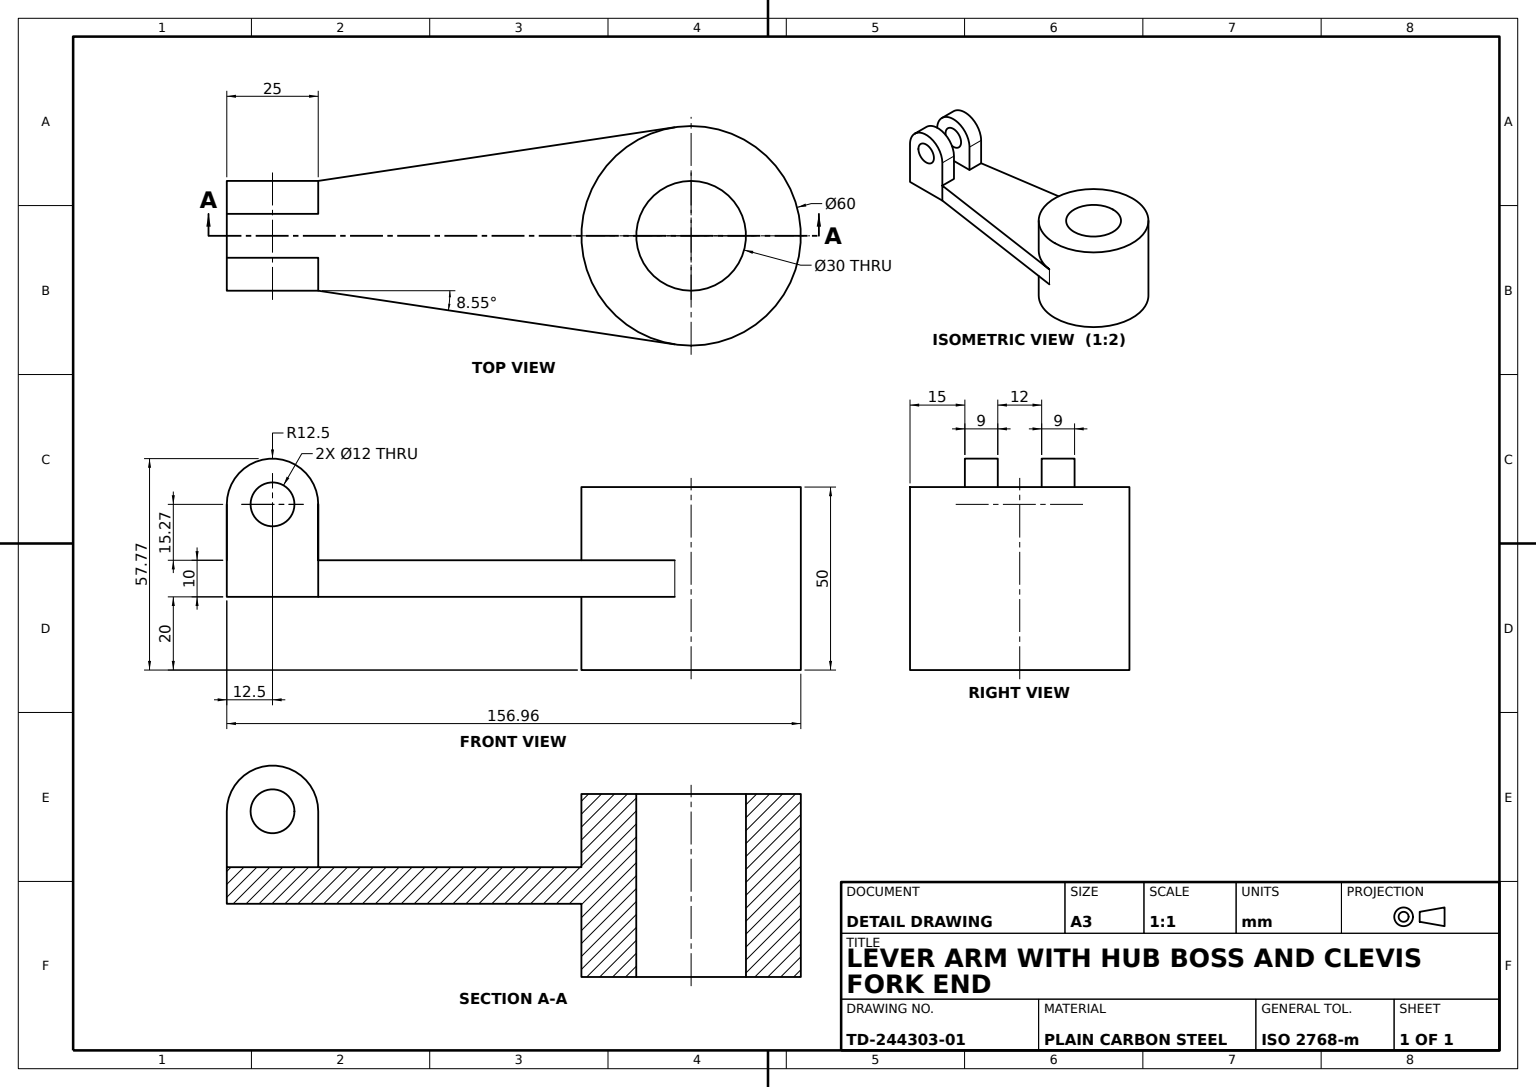
SolidWorks part; units mm, degrees
material "Plain Carbon Steel"
ref_plane "Front Plane" through (0, 0, 0) normal (0, 0, 1) x (1, 0, 0)
ref_plane "Top Plane" through (0, 0, 0) normal (0, 1, 0) x (1, 0, 0)
ref_plane "Right Plane" through (0, 0, 0) normal (1, 0, 0) x (0, 0, -1)
sketch "Hub Sketch Ø60" plane through (0, 0, 0) normal (0, 1, 0) x (1, 0, 0)
  circle A0 centre (0, 0) radius 30
  dimension "D1" = 60
extrude "Hub Ø60x50" add sketch "Hub Sketch Ø60" along normal mid plane 50
sketch "Bore Sketch Ø30" plane through (0, 25, 0) normal (0, 1, 0) x (1, 0, 0)
  circle A0 centre (0, 0) radius 15
  dimension "D1" = 30
extrude "Hub Bore Ø30" cut sketch "Bore Sketch Ø30" against normal through all contours A0
sketch "Arm Plate Sketch" plane through (0, 0, 0) normal (0, 1, 0) x (1, 0, 0)
  line L0 (-101.9625, 15) -> (-4.4625, 29.6662)
  line L1 (-101.9625, -15) -> (-4.4625, -29.6662)
  line L2 (-101.9625, -15) -> (-101.9625, 15)
  arc A0 (-4.4625, 29.6662) -> (-4.4625, -29.6662) centre (0, 0) ccw
  dimension "D1" = 60
  dimension "D2" = 97.5
  dimension "D3" = 30
  dimension "D4" = 97.5
extrude "Arm Plate 10mm" add sketch "Arm Plate Sketch" along normal mid plane 10 contours L2 L0 A0 L1
sketch "Clevis Base Sketch" plane through (0, 5, 0) normal (0, 1, 0) x (1, 0, 0)
  line L0 (-101.9625, -15) -> (-126.9625, -15)
  line L1 (-126.9625, -15) -> (-126.9625, 15)
  line L2 (-101.9625, 15) -> (-126.9625, 15)
  line L6 (-101.9625, -15) -> (-4.4625, -29.6662)
  line L7 (-4.4625, 29.6662) -> (-101.9625, 15)
  line L8 (-101.9625, 15) -> (-101.9625, -15)
  line L9 (-101.9625, -15) -> (-4.4625, -29.6662)
  line L10 (-4.4625, 29.6662) -> (-101.9625, 15)
  arc A1 (-4.4625, 29.6662) -> (-4.4625, -29.6662) centre (0, 0) ccw
  arc A2 (-4.4625, 29.6662) -> (-4.4625, -29.6662) centre (0, 0) ccw
  dimension "D1" = 25
  dimension "D2" = 0
extrude "Clevis Base" add sketch "Clevis Base Sketch" against normal blind 10 contours L0 L1 L2 L10 A2 L9
sketch "Clevis Lug 1 Sketch" plane through (0, 0, 15) normal (0, 0, 1) x (1, 0, 0)
  line L0 (-101.9625, 5) -> (-101.9625, 20.2721)
  line L1 (-126.9625, -5) -> (-126.9625, 5) construction
  line L2 (-126.9625, 20.2721) -> (-126.9625, 5)
  line L4 (-101.9625, 5) -> (-126.9625, 5) construction
  arc A0 (-101.9625, 20.2721) -> (-126.9625, 20.2721) centre (-114.4625, 20.2721) ccw
  circle A1 centre (-114.4625, 20.2721) radius 6
  line M1 (-101.9625, 5) -> (-126.9625, 5)
  dimension "D1" = 12
  dimension "D2" = 15.2721
extrude "Clevis Lug 1" add sketch "Clevis Lug 1 Sketch" against normal blind 9 contours L0 A0 L2 A1 M1
sketch "Clevis Lug 2 Sketch" plane through (0, 0, -15) normal (0, 0, -1) x (-1, 0, 0)
  line L0 (101.9625, 5) -> (101.9625, 20.2721) construction
  line L1 (101.9625, 5) -> (101.9625, 20.2721)
  line L2 (126.9625, 20.2721) -> (126.9625, 5) construction
  line L3 (126.9625, 20.2721) -> (126.9625, 5)
  arc A0 (126.9625, 20.2721) -> (101.9625, 20.2721) centre (114.4625, 20.2721) ccw construction
  arc A1 (126.9625, 20.2721) -> (101.9625, 20.2721) centre (114.4625, 20.2721) ccw
  circle A2 centre (114.4625, 20.2721) radius 6 construction
  circle A3 centre (114.4625, 20.2721) radius 6
  line M5 (126.9625, 5) -> (101.9625, 5)
extrude "Clevis Lug 2" add sketch "Clevis Lug 2 Sketch" against normal blind 9 contours L3 A1 L1 A3 M5
